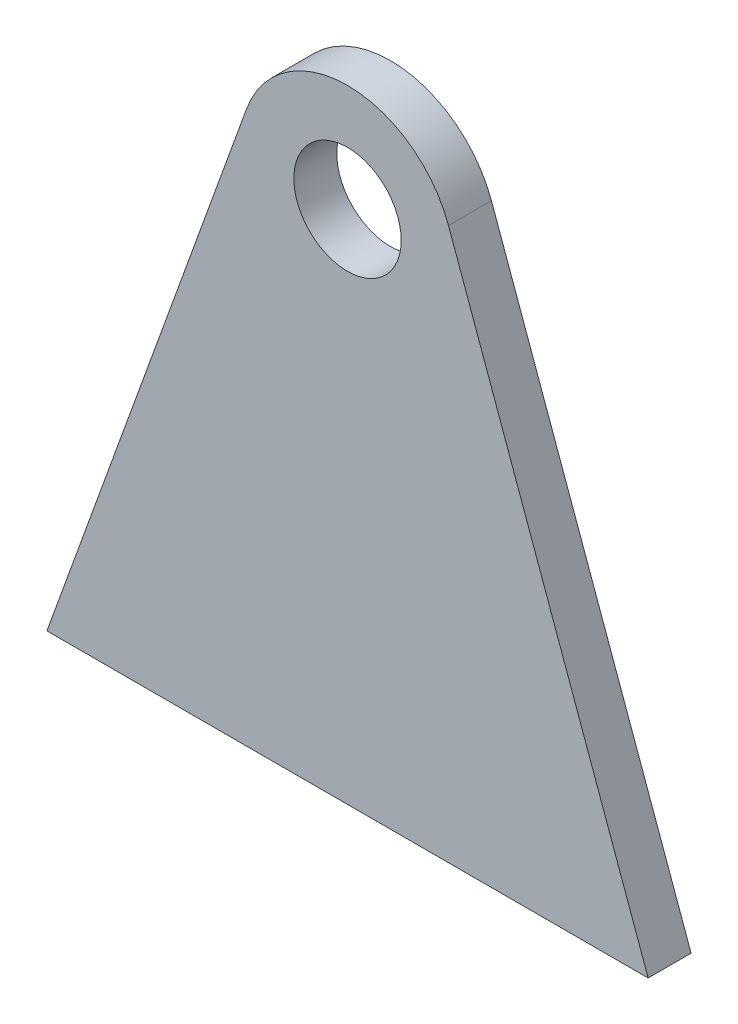
from build123d import *

# Parameters (mm, degrees)
LUG_PROFILE_SKETCH_R = 25
LUG_PLATE_20MM_DEPTH = 20


with BuildPart() as part:
    # Lug Profile Sketch → Lug Plate 20mm (new body)
    with BuildSketch(Plane.XY):
        with BuildLine():
            Line((-140, -240), (140, -240))
            Line((140, -240), (47.017565913, 17.010246783))
            ThreePointArc((47.017565913, 17.010246783), (0, 50), (-47.017565913, 17.010246783))
            Line((-47.017565913, 17.010246783), (-140, -240))
        make_face()
        Circle(LUG_PROFILE_SKETCH_R, mode=Mode.SUBTRACT)
    extrude(amount=LUG_PLATE_20MM_DEPTH)


solid = part.part
